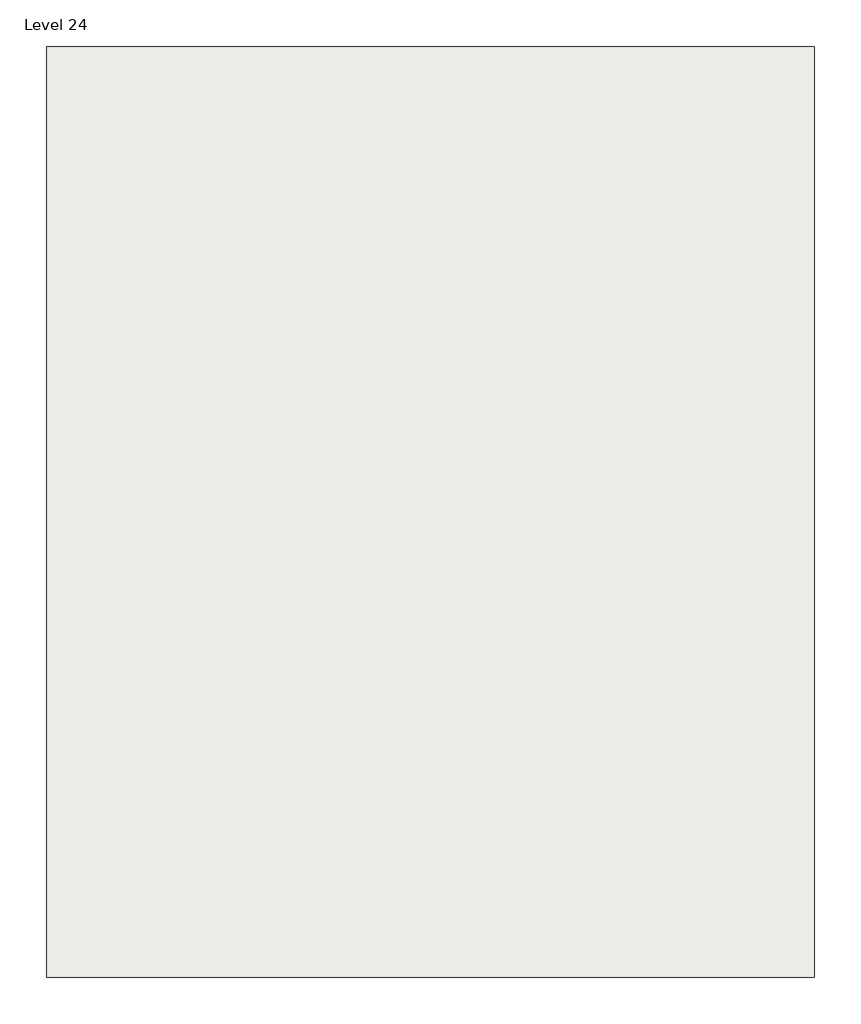
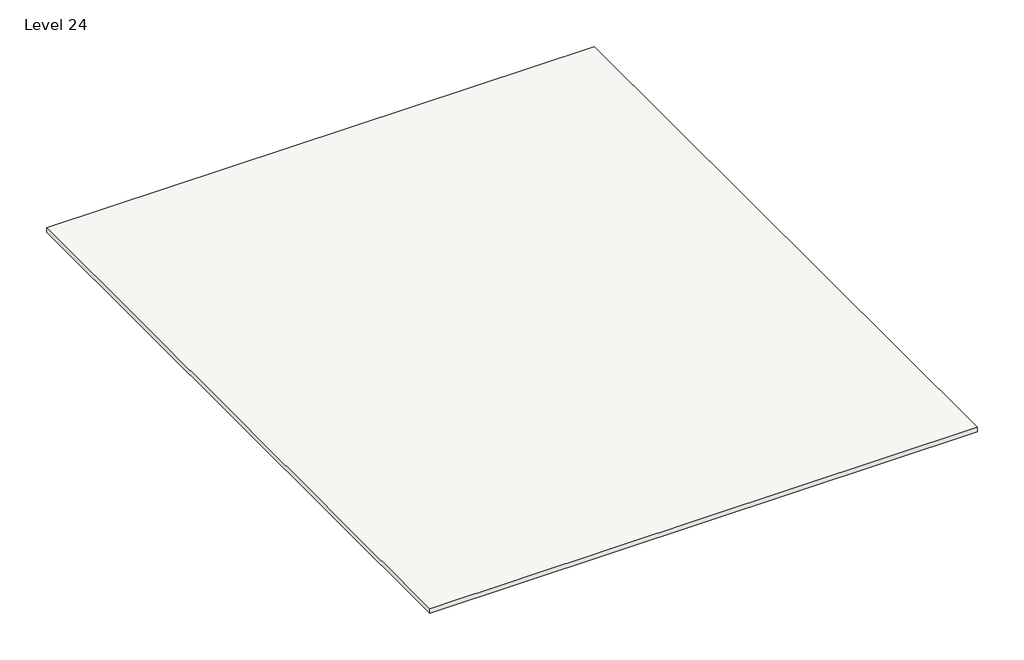
# One storey: 1 slab.
"""IFC4 building model written with IfcOpenShell, lengths in millimetres."""

from ifc_helpers import new_model, si_unit, frame, origin, place, context, project, spatial, polyline, outline, extrude, element, save

model = new_model("IFC4")

# Units and contexts
model_context = context("Model", 3, world=origin())
ifc_project = project(units=[si_unit("LENGTHUNIT", "METRE", prefix="MILLI")], contexts=[model_context])

# Site, building, storey
site = spatial("IfcSite", under=ifc_project)
building = spatial("IfcBuilding", under=site)
storey = spatial("IfcBuildingStorey", under=building, Name="Level 24", Elevation=39624.0)

# Slab
placement = place(None, origin())
element("IfcSlab", 1, ObjectType="Generic - 12\"", at=placement, inside=storey, context=model_context, shape_type="SweptSolid", body=[
    extrude(outline(polyline([(19165.761926, 20708.4177494), (19165.761926, -21049.1822506), (-15276.638074, -21049.1822506), (-15276.638074, 20708.4177494), (19165.761926, 20708.4177494)])), frame((0.0, 0.0, 39560.282979), z_axis=(0.0, 0.0, 1.0), x_axis=(1.0, 0.0, 0.0)), (0.0, 0.0, 1.0), 304.8),
])

save(model, "model.ifc")

# Revit data of these elements
# Type "Generic - 12\""
#   Assembly Code = "B1010"
#   Function = 0
#   Layers, outside or top first: 1' - 0" no material (function 1)
# Element 1 (IfcSlab, "Generic - 12\"")
#   Height Offset From Level = 0' - 9.49146"
#   Phase Created = New Construction
#   Materials on its faces: "Default Floor"
# Materials
#   "Default Floor": colour RGB 128 128 128, transparency 0
